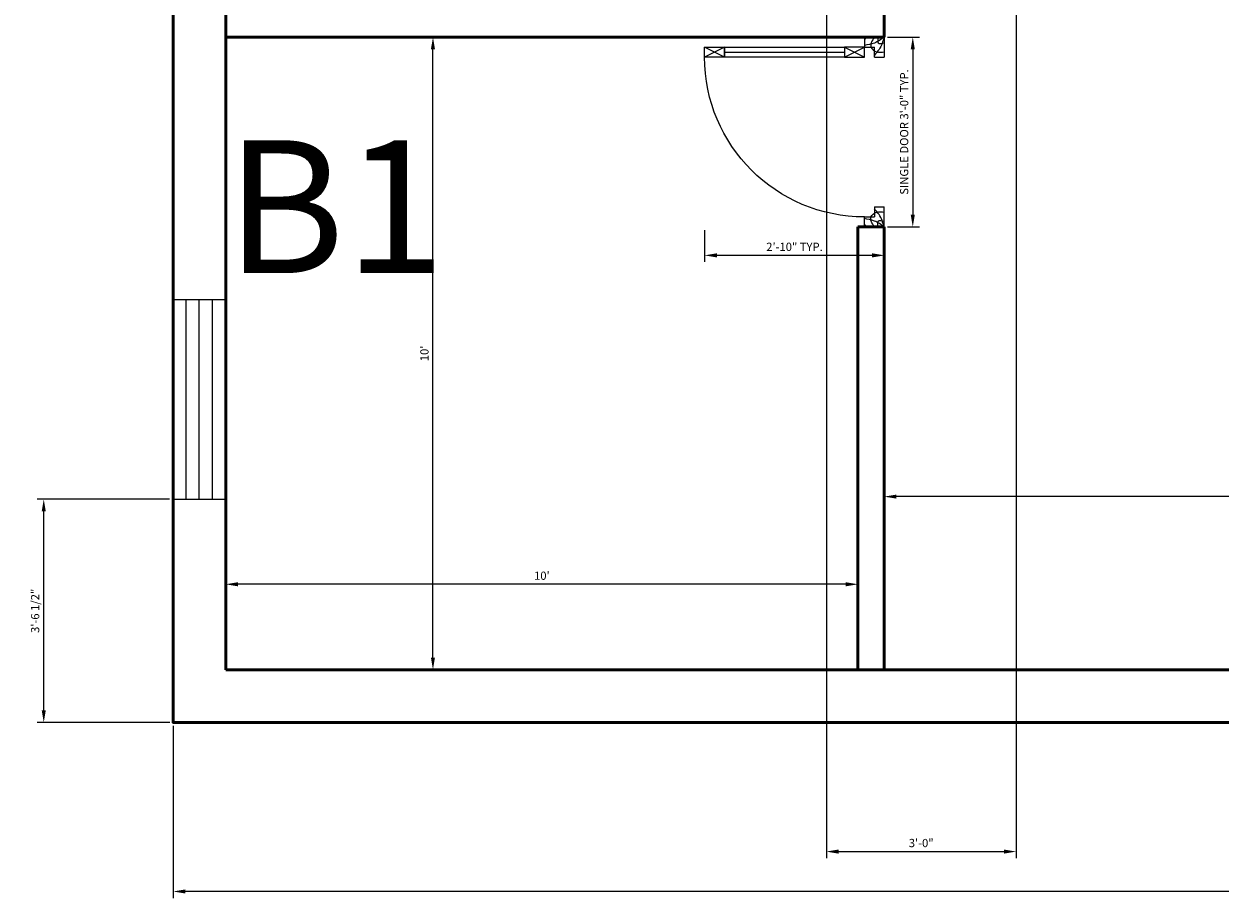
# Model space of a CAD drawing. Units: inches. Extents: x -28 to 484, y -33 to 391.
# Tile 1 of 4: x -28 to 199, y -33 to 133. Entities that reach past the tile are written whole.
import ezdxf

# ---------------------------------------------------------------- set-up
doc = ezdxf.new("R2010")
doc.units = ezdxf.units.IN
for name, color, linetype, lineweight in [('A-ANNO-DIMS', 2, 'Continuous', 18), ('A-AREA-IDEN', 7, 'Continuous', 25), ('A-DOOR', 3, 'Continuous', 25), ('A-GLAZ', 4, 'Continuous', 18), ('A-WALL', 7, 'Continuous', 50)]:
    doc.layers.add(name, color=color, linetype=linetype, lineweight=lineweight)
doc.styles.get("Standard").update_dxf_attribs({"font": 'arial.ttf'})
doc.dimstyles.new('ISO-25', dxfattribs={"dimtxt": 1.5625, "dimasz": 2.3125, "dimexe": 1.25, "dimexo": 0.625, "dimtad": 1, "dimlunit": 4, "dimtxsty": 'Standard', "dimcen": 2.5, "dimadec": 0, "dimazin": 0, "dimtfac": 1, "dimtmove": 0, "dimatfit": 3, "dimfxl": 1, "dimarcsym": 0})

# ---------------------------------------------------------------- blocks, each defined once
blk = doc.blocks.new('A$C05E21637')
for p, q in [((50, 800), (100, 900)), ((100, 800), (50, 900)), ((75, 800), (75, 200)), ((100, 200), (50, 100)), ((50, 200), (100, 100)), ((0, 100), (0, 0)), ((0, 100), (50, 100)), ((50, 100), (50, 50)), ((900, 100), (900, 50)), ((950, 100), (900, 100)), ((950, 100), (950, 0)), ((100, 50), (50, 50)), ((100, 50), (100, 0)), ((850, 50), (900, 50)), ((850, 50), (850, 0)), ((0, 0), (100, 0)), ((950, 0), (850, 0))]:
    blk.add_line(p, q)
for points in [[(50, 800), (100, 800), (100, 900), (50, 900)], [(50, 200), (100, 200), (100, 800), (50, 800)], [(50, 200), (100, 200), (100, 100), (50, 100)]]:
    blk.add_lwpolyline(points, close=True)
blk.add_arc((100, 100), 800, 0, 90)
for points, knots in [([(0, 0), (11.2, 16), (32.5, 46.3), (38.7, 82.7), (41.2, 100)], [0, 0, 0, 0, 57.729567, 109.527977, 109.527977, 109.527977, 109.527977]), ([(0, 50), (17.5, 61.3), (46.9, 80.3), (79.6, 38.4), (75.6, 13.1), (73.5, 0)], [0, 0, 0, 0, 52.797078, 89.119952, 128.374378, 128.374378, 128.374378, 128.374378]), ([(950, 50), (932.5, 61.3), (903.1, 80.3), (870.4, 38.4), (874.4, 13.1), (876.5, 0)], [0, 0, 0, 0, 52.797078, 89.119952, 128.374378, 128.374378, 128.374378, 128.374378]), ([(950, 0), (938.8, 16), (917.5, 46.3), (911.3, 82.7), (908.8, 100)], [0, 0, 0, 0, 57.729567, 109.527977, 109.527977, 109.527977, 109.527977]), ([(0, 0), (21.6, 7.2), (55.2, 18.3), (81.2, 41.3), (90.1, 50)], [0, 0, 0, 0, 67.133415, 104.197904, 104.197904, 104.197904, 104.197904]), ([(0, 30.3), (11.9, 32.6), (36.4, 37.4), (31.4, 12.7), (28.8, 0)], [0, 0, 0, 0, 28.773527, 59.024697, 59.024697, 59.024697, 59.024697]), ([(950, 0), (928.4, 7.2), (894.8, 18.3), (868.8, 41.3), (859.9, 50)], [0, 0, 0, 0, 67.133415, 104.197904, 104.197904, 104.197904, 104.197904]), ([(950, 30.3), (938.1, 32.6), (913.6, 37.4), (918.6, 12.7), (921.2, 0)], [0, 0, 0, 0, 28.773527, 59.024697, 59.024697, 59.024697, 59.024697])]:
    blk.add_open_spline(points, degree=3, knots=knots)
for points in [[(0, 86.7), (4.7, 91.3), (9.4, 95.9), (15.1, 100)], [(950, 86.7), (945.3, 91.3), (940.6, 95.9), (934.9, 100)]]:
    blk.add_open_spline(points, degree=3)
blk = doc.blocks.new('*D10')
at = {"layer": 'A-ANNO-DIMS', "color": 0, "lineweight": -2, "transparency": 16777216}
for p, q in [((135, 51.37), (135, 41.58)), ((297, 51.37), (297, 41.58)), ((294.69, 42.83), (137.31, 42.83))]:
    blk.add_line(p, q, dxfattribs=at)
at = {"layer": 'A-ANNO-DIMS', "color": 0, "transparency": 16777216}
for points in [[(137.31, 43.22), (137.31, 42.45), (135, 42.83)], [(294.69, 43.22), (294.69, 42.45), (297, 42.83)]]:
    blk.add_solid(points, dxfattribs=at)
at = {"layer": 'Defpoints', "color": 0, "transparency": 16777216}
for p in [(135, 52), (297, 52), (135, 42.83)]:
    blk.add_point(p, dxfattribs=at)
at = {"layer": 'A-ANNO-DIMS', "color": 0, "transparency": 16777216, "insert": (216, 44.26), "char_height": 1.562, "attachment_point": 5}
blk.add_mtext('13\'-6"', dxfattribs=at)
blk = doc.blocks.new('*D11')
at = {"layer": 'A-ANNO-DIMS', "color": 0, "lineweight": -2, "transparency": 16777216}
for p, q in [((10, 30.57), (10, 24.96)), ((130, 30.57), (130, 24.96)), ((127.69, 26.21), (12.31, 26.21))]:
    blk.add_line(p, q, dxfattribs=at)
at = {"layer": 'A-ANNO-DIMS', "color": 0, "transparency": 16777216}
for points in [[(12.31, 26.59), (12.31, 25.82), (10, 26.21)], [(127.69, 26.59), (127.69, 25.82), (130, 26.21)]]:
    blk.add_solid(points, dxfattribs=at)
at = {"layer": 'Defpoints', "color": 0, "transparency": 16777216}
for p in [(10, 31.19), (130, 31.19), (10, 26.21)]:
    blk.add_point(p, dxfattribs=at)
at = {"layer": 'A-ANNO-DIMS', "color": 0, "transparency": 16777216, "insert": (70, 27.63), "char_height": 1.562, "attachment_point": 5}
blk.add_mtext("10'", dxfattribs=at)
blk = doc.blocks.new('*D12')
at = {"layer": 'A-ANNO-DIMS', "color": 0, "lineweight": -2, "transparency": 16777216}
for p, q in [((49.05, 130), (50.58, 130)), ((49.33, 12.31), (49.33, 127.69)), ((42.7, 10), (50.58, 10))]:
    blk.add_line(p, q, dxfattribs=at)
at = {"layer": 'A-ANNO-DIMS', "color": 0, "transparency": 16777216}
for points in [[(48.94, 127.69), (49.71, 127.69), (49.33, 130)], [(48.94, 12.31), (49.71, 12.31), (49.33, 10)]]:
    blk.add_solid(points, dxfattribs=at)
at = {"layer": 'Defpoints', "color": 0, "transparency": 16777216}
for p in [(48.42, 130), (49.33, 130), (42.07, 10)]:
    blk.add_point(p, dxfattribs=at)
at = {"layer": 'A-ANNO-DIMS', "color": 0, "transparency": 16777216, "insert": (47.91, 70), "char_height": 1.562, "attachment_point": 5, "rotation": 90}
blk.add_mtext("10'", dxfattribs=at)
blk = doc.blocks.new('*D18')
at = {"layer": 'A-ANNO-DIMS', "color": 0, "lineweight": -2, "transparency": 16777216}
for p, q in [((0, -0.62), (0, -33.32)), ((456, -0.62), (456, -33.32)), ((453.69, -32.07), (2.31, -32.07))]:
    blk.add_line(p, q, dxfattribs=at)
at = {"layer": 'A-ANNO-DIMS', "color": 0, "transparency": 16777216}
for points in [[(2.31, -31.68), (2.31, -32.45), (0, -32.07)], [(453.69, -31.68), (453.69, -32.45), (456, -32.07)]]:
    blk.add_solid(points, dxfattribs=at)
at = {"layer": 'Defpoints', "color": 0, "transparency": 16777216}
for p in [(0, 0), (456, 0), (0, -32.07)]:
    blk.add_point(p, dxfattribs=at)
at = {"layer": 'A-ANNO-DIMS', "color": 0, "transparency": 16777216, "insert": (228, -30.64), "char_height": 1.562, "attachment_point": 5}
blk.add_mtext("38'", dxfattribs=at)
blk = doc.blocks.new('WIN-PLAN-FRAME')
for p, q in [((0, 10), (0, 0)), ((37.87, 10), (37.87, 0)), ((0, 7.5), (37.87, 7.5)), ((0, 5), (37.87, 5)), ((0, 2.5), (37.87, 2.5))]:
    blk.add_line(p, q)
blk = doc.blocks.new('*D20')
at = {"layer": 'A-ANNO-DIMS', "color": 0, "lineweight": -2, "transparency": 16777216}
for p, q in [((135.62, 130), (141.65, 130)), ((140.4, 127.69), (140.4, 96.31)), ((135.62, 94), (141.65, 94))]:
    blk.add_line(p, q, dxfattribs=at)
at = {"layer": 'A-ANNO-DIMS', "color": 0, "transparency": 16777216}
for points in [[(140.01, 127.69), (140.79, 127.69), (140.4, 130)], [(140.01, 96.31), (140.79, 96.31), (140.4, 94)]]:
    blk.add_solid(points, dxfattribs=at)
at = {"layer": 'Defpoints', "color": 0, "transparency": 16777216}
for p in [(135, 130), (135, 94), (140.4, 94)]:
    blk.add_point(p, dxfattribs=at)
at = {"layer": 'A-ANNO-DIMS', "color": 0, "transparency": 16777216, "insert": (138.97, 112), "char_height": 1.5625, "attachment_point": 5, "rotation": 90}
blk.add_mtext('SINGLE DOOR 3\'-0" TYP.', dxfattribs=at)
blk = doc.blocks.new('*D21')
at = {"layer": 'A-ANNO-DIMS', "color": 0, "lineweight": -2, "transparency": 16777216}
for p, q in [((100.89, 93.37), (100.89, 87.35)), ((135, 93.37), (135, 87.35)), ((132.69, 88.6), (103.21, 88.6))]:
    blk.add_line(p, q, dxfattribs=at)
at = {"layer": 'A-ANNO-DIMS', "color": 0, "transparency": 16777216}
for points in [[(103.21, 88.99), (103.21, 88.21), (100.89, 88.6)], [(132.69, 88.99), (132.69, 88.21), (135, 88.6)]]:
    blk.add_solid(points, dxfattribs=at)
at = {"layer": 'Defpoints', "color": 0, "transparency": 16777216}
for p in [(100.89, 94), (135, 94), (100.89, 88.6)]:
    blk.add_point(p, dxfattribs=at)
at = {"layer": 'A-ANNO-DIMS', "color": 0, "transparency": 16777216, "insert": (117.95, 90.02), "char_height": 1.5625, "attachment_point": 5}
blk.add_mtext('2\'-10" TYP.', dxfattribs=at)
blk = doc.blocks.new('*D32')
at = {"layer": 'A-ANNO-DIMS', "color": 0, "lineweight": -2, "transparency": 16777216}
for p, q in [((-0.67, 42.34), (-25.8, 42.34)), ((-24.55, 2.31), (-24.55, 40.03)), ((-0.63, 0), (-25.8, 0))]:
    blk.add_line(p, q, dxfattribs=at)
at = {"layer": 'A-ANNO-DIMS', "color": 0, "transparency": 16777216}
for points in [[(-24.93, 40.03), (-24.16, 40.03), (-24.55, 42.34)], [(-24.93, 2.31), (-24.16, 2.31), (-24.55, 0)]]:
    blk.add_solid(points, dxfattribs=at)
at = {"layer": 'Defpoints', "color": 0, "transparency": 16777216}
for p in [(-24.55, 42.34), (-0.05, 42.34), (0, 0)]:
    blk.add_point(p, dxfattribs=at)
at = {"layer": 'A-ANNO-DIMS', "color": 0, "transparency": 16777216, "insert": (-25.98, 21.17), "char_height": 1.562, "attachment_point": 5, "rotation": 90}
blk.add_mtext('3\'-6 1/2"', dxfattribs=at)
blk = doc.blocks.new('*D36')
at = {"layer": 'A-ANNO-DIMS', "color": 0, "lineweight": -2, "transparency": 16777216}
for p, q in [((124, 261.38), (124, -25.75)), ((160, 261.38), (160, -25.75)), ((126.31, -24.5), (157.69, -24.5))]:
    blk.add_line(p, q, dxfattribs=at)
at = {"layer": 'A-ANNO-DIMS', "color": 0, "transparency": 16777216}
for points in [[(126.31, -24.11), (126.31, -24.89), (124, -24.5)], [(157.69, -24.11), (157.69, -24.89), (160, -24.5)]]:
    blk.add_solid(points, dxfattribs=at)
at = {"layer": 'Defpoints', "color": 0, "transparency": 16777216}
for p in [(124, 262), (160, 262), (160, -24.5)]:
    blk.add_point(p, dxfattribs=at)
at = {"layer": 'A-ANNO-DIMS', "color": 0, "transparency": 16777216, "insert": (142, -23.08), "char_height": 1.562, "attachment_point": 5}
blk.add_mtext('3\'-0"', dxfattribs=at)

msp = doc.modelspace()

# ---------------------------------------------------------------- linework, layer by layer
at = {"layer": 'A-WALL'}
for p, q in [((10, 258), (10, 10)), ((135, 135), (135, 130)), ((10, 130), (135, 130)), ((130, 94), (130, 10)), ((130, 94), (135, 94)), ((135, 94), (135, 10)), ((10, 10), (446, 10))]:
    msp.add_line(p, q, dxfattribs=at)
msp.add_lwpolyline([(0, 258), (0, 0), (456, 0), (456, 342), (0, 342)], dxfattribs=at)

# ---------------------------------------------------------------- block references
at = {"layer": 'A-DOOR', "xscale": -0.0378947368421072, "yscale": 0.0378947368421072, "zscale": 0.0378947368421072, "rotation": 89.99999999998745}
msp.add_blockref('A$C05E21637', (135, 130), dxfattribs=at)
at = {"layer": 'A-GLAZ', "rotation": 90.00000000000006}
msp.add_blockref('WIN-PLAN-FRAME', (9.954, 42.342), dxfattribs=at)

# ---------------------------------------------------------------- texts
at = {"layer": 'A-AREA-IDEN', "insert": (10, 110.434), "char_height": 25.2055, "attachment_point": 1}
msp.add_mtext_dynamic_manual_height_columns('B1', width=32.60059, gutter_width=126.027, heights=[0], dxfattribs=at)

# ---------------------------------------------------------------- dimensions: what is measured, and where the dimension line sits
at = {"layer": 'A-ANNO-DIMS'}
for base, p1, p2, override, picture, middle in [((160, -24.5), (124, 262), (160, 262), {"dimdec": 1, "dimlfac": 1, "dimrnd": 0, "dimzin": 1, "dimdsep": 46, "dimlunit": 4, "dimfrac": 2}, '*D36', (142, -23.077)), ((135, 42.833), (297, 52), (135, 52), {"dimclrd": 0, "dimclre": 0, "dimclrt": 0}, '*D10', (216, 44.257)), ((10, 26.206), (130, 31.192), (10, 31.192), {"dimclrd": 0, "dimclre": 0, "dimclrt": 0}, '*D11', (70, 27.629)), ((0, -32.067), (456, 0), (0, 0), {"dimclrd": 0, "dimclre": 0, "dimclrt": 0}, '*D18', (228, -30.644))]:
    dim = msp.add_linear_dim(base=base, p1=p1, p2=p2, dimstyle='ISO-25', override=override, dxfattribs=at)
    dim.commit()
    dim.dimension.update_dxf_attribs({"geometry": picture, "text_midpoint": middle})
for base, p1, p2, override, picture, middle in [((49.329, 130), (42.071, 10), (48.422, 130), {"dimclrd": 0, "dimclre": 0, "dimclrt": 0}, '*D12', (47.906, 70)), ((-24.546, 42.342), (0, 0), (-0.046, 42.342), {"dimdec": 1, "dimlfac": 1, "dimrnd": 0, "dimzin": 1, "dimdsep": 46, "dimlunit": 4, "dimfrac": 2}, '*D32', (-25.979, 21.171))]:
    dim = msp.add_linear_dim(base=base, p1=p1, p2=p2, angle=90, dimstyle='ISO-25', override=override, dxfattribs=at)
    dim.commit()
    dim.dimension.update_dxf_attribs({"geometry": picture, "text_midpoint": middle})
for base, p1, p2, angle, text, picture, middle in [((140.4, 94), (135, 130), (135, 94), 270, 'SINGLE DOOR <> TYP.', '*D20', (138.966, 112)), ((100.895, 88.6), (135, 94), (100.895, 94), 180, '<> TYP.', '*D21', (117.947, 90.023))]:
    dim = msp.add_linear_dim(base=base, p1=p1, p2=p2, angle=angle, text=text, dimstyle='ISO-25', override={"dimdec": 1, "dimlfac": 1, "dimrnd": 0, "dimzin": 1, "dimdsep": 46, "dimlunit": 4, "dimfrac": 2}, dxfattribs=at)
    dim.commit()
    dim.dimension.update_dxf_attribs({"geometry": picture, "text_midpoint": middle})

doc.saveas('drawing.dxf')
